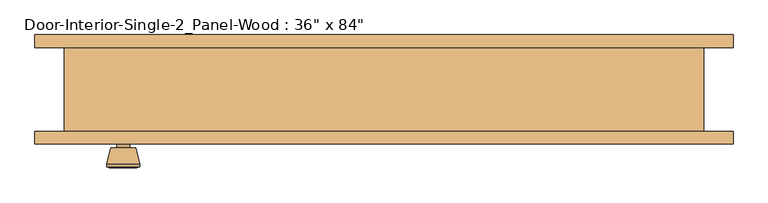
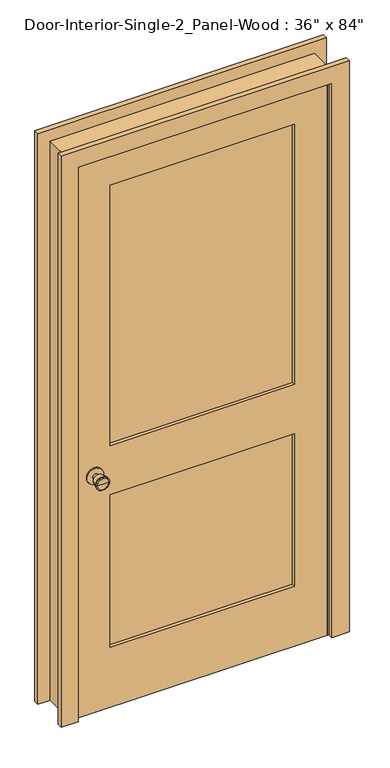
"""IFC4 building model written with IfcOpenShell, lengths in millimetres: door geometry."""

from ifc_helpers import new_model, si_unit, point, frame, frame_2d, origin, place, context, project, spatial, polyline, circle_curve, trimmed, segment, composite_curve, outline, extrude, faceted_brep, source, transform, mapped, element, save
from ifc_brep_helpers import plane_surface, cylinder_surface, revolved_surface, advanced_brep


def door_2e56f206(model_context):
    return source(origin(), model_context, "Body", "SolidModel", [
        advanced_brep(
        [(-393.7, -19.4, 914.4), (-403.7, -19.4, 914.4), (-383.7, -19.4, 914.4), (-373.2241324, 29.6, 914.4), (-414.1758676, 29.6, 914.4), (-393.7, 29.6, 914.4), (-368.7, 27.7721319, 914.4), (-418.7, 27.7721319, 914.4), (-368.7, 24.3084537, 914.4), (-418.7, 24.3084537, 914.4), (-375.063764, -0.4, 914.4), (-412.336236, -0.4, 914.4), (-383.7, -0.4, 914.4), (-403.7, -0.4, 914.4)],
        [
            (0, 1),
            (1, 2, circle_curve(frame((-393.7, -19.4, 914.4), z_axis=(0.0, -1.0, 0.0), x_axis=(-1.0, 0.0, 0.0)), 10.0)),
            (2, 0),
            (2, 1, circle_curve(frame((-393.7, -19.4, 914.4), z_axis=(0.0, -1.0, 0.0), x_axis=(-1.0, 0.0, 0.0)), 10.0)),
            (3, 4, circle_curve(frame((-393.7, 29.6, 914.4), z_axis=(0.0, 1.0, 0.0), x_axis=(-1.0, 0.0, 0.0)), 20.4758676)),
            (4, 5),
            (5, 3),
            (4, 3, circle_curve(frame((-393.7, 29.6, 914.4), z_axis=(0.0, 1.0, 0.0), x_axis=(-1.0, 0.0, 0.0)), 20.4758676)),
            (6, 7, circle_curve(frame((-393.7, 27.7721319, 914.4), z_axis=(0.0, 1.0, 0.0), x_axis=(-1.0, 0.0, 0.0)), 25.0)),
            (7, 4),
            (3, 6),
            (7, 6, circle_curve(frame((-393.7, 27.7721319, 914.4), z_axis=(0.0, 1.0, 0.0), x_axis=(-1.0, 0.0, 0.0)), 25.0)),
            (8, 9, circle_curve(frame((-393.7, 24.3084537, 914.4), z_axis=(0.0, 1.0, 0.0), x_axis=(-1.0, 0.0, 0.0)), 25.0)),
            (9, 7),
            (6, 8),
            (9, 8, circle_curve(frame((-393.7, 24.3084537, 914.4), z_axis=(0.0, 1.0, 0.0), x_axis=(-1.0, 0.0, 0.0)), 25.0)),
            (10, 11, circle_curve(frame((-393.7, -0.4, 914.4), z_axis=(0.0, 1.0, 0.0), x_axis=(-1.0, 0.0, 0.0)), 18.636236)),
            (11, 9),
            (8, 10),
            (11, 10, circle_curve(frame((-393.7, -0.4, 914.4), z_axis=(0.0, 1.0, 0.0), x_axis=(-1.0, 0.0, 0.0)), 18.636236)),
            (12, 13, circle_curve(frame((-393.7, -0.4, 914.4), z_axis=(0.0, 1.0, 0.0), x_axis=(-1.0, 0.0, 0.0)), 10.0)),
            (13, 11),
            (10, 12),
            (13, 12, circle_curve(frame((-393.7, -0.4, 914.4), z_axis=(0.0, 1.0, 0.0), x_axis=(-1.0, 0.0, 0.0)), 10.0)),
            (1, 13),
            (12, 2),
        ],
        [
            plane_surface(frame((-393.7, -19.4, 914.4), z_axis=(0.0, -1.0, 0.0), x_axis=(-1.0, 0.0, 0.0))),
            plane_surface(frame((-393.7, 29.6, 914.4), z_axis=(0.0, 1.0, 0.0), x_axis=(-1.0, 0.0, 0.0))),
            revolved_surface(polyline([(-414.1758676, 29.6, 914.4), (-418.7, 27.7721319, 914.4)]), (-393.7, -19.4, 914.4), (0.0, -1.0, 0.0)),
            cylinder_surface(frame((-393.7, -19.4, 914.4), z_axis=(0.0, -1.0, 0.0), x_axis=(-1.0, 0.0, 0.0)), 25.0),
            revolved_surface(polyline([(-418.7, 24.3084537, 914.4), (-412.336236, -0.4, 914.4)]), (-393.7, -19.4, 914.4), (0.0, -1.0, 0.0)),
            plane_surface(frame((-393.7, -0.4, 914.4), z_axis=(0.0, -1.0, 0.0), x_axis=(-1.0, 0.0, 0.0))),
            cylinder_surface(frame((-393.7, -19.4, 914.4), z_axis=(0.0, -1.0, 0.0), x_axis=(-1.0, 0.0, 0.0)), 10.0),
        ],
        [
            (0, [[1, 2, 3]]),
            (0, [[-3, 4, -1]]),
            (1, [[5, 6, 7]]),
            (1, [[8, -7, -6]]),
            (2, [[9, 10, -5, 11]]),
            (2, [[12, -11, -8, -10]]),
            (3, [[13, 14, -9, 15]]),
            (3, [[16, -15, -12, -14]]),
            (4, [[17, 18, -13, 19]]),
            (4, [[20, -19, -16, -18]]),
            (5, [[21, 22, -17, 23]]),
            (5, [[24, -23, -20, -22]]),
            (6, [[-2, 25, -21, 26]]),
            (6, [[-4, -26, -24, -25]]),
        ],
    ),
        extrude(outline(composite_curve([segment(trimmed(circle_curve(frame_2d((914.4, -393.7)), 30.0), [point((914.4, -423.7))], [point((914.4, -363.7))], False, "CARTESIAN"), True, "CONTINUOUS"), segment(trimmed(circle_curve(frame_2d((914.4, -393.7)), 30.0), [point((914.4, -363.7))], [point((914.4, -423.7))], False, "CARTESIAN"), True, "CONTINUOUS")], self_intersect=False)), frame((0.0, -25.4, 0.0), z_axis=(0.0, 1.0, 0.0), x_axis=(0.0, 0.0, 1.0)), (0.0, 0.0, 1.0), 6.0),
        advanced_brep(
        [(-393.7, -66.325, 914.4), (-383.7, -66.325, 914.4), (-403.7, -66.325, 914.4), (-373.2241324, -115.325, 914.4), (-393.7, -115.325, 914.4), (-414.1758676, -115.325, 914.4), (-368.7, -113.4971319, 914.4), (-418.7, -113.4971319, 914.4), (-368.7, -110.0334537, 914.4), (-418.7, -110.0334537, 914.4), (-375.063764, -85.325, 914.4), (-412.336236, -85.325, 914.4), (-383.7, -85.325, 914.4), (-403.7, -85.325, 914.4)],
        [
            (0, 1),
            (1, 2, circle_curve(frame((-393.7, -66.325, 914.4), z_axis=(0.0, 1.0, 0.0), x_axis=(-1.0, 0.0, 0.0)), 10.0)),
            (2, 0),
            (2, 1, circle_curve(frame((-393.7, -66.325, 914.4), z_axis=(0.0, 1.0, 0.0), x_axis=(-1.0, 0.0, 0.0)), 10.0)),
            (3, 4),
            (4, 5),
            (5, 3, circle_curve(frame((-393.7, -115.325, 914.4), z_axis=(0.0, -1.0, 0.0), x_axis=(-1.0, 0.0, 0.0)), 20.4758676)),
            (3, 5, circle_curve(frame((-393.7, -115.325, 914.4), z_axis=(0.0, -1.0, 0.0), x_axis=(-1.0, 0.0, 0.0)), 20.4758676)),
            (6, 3),
            (5, 7),
            (7, 6, circle_curve(frame((-393.7, -113.4971319, 914.4), z_axis=(0.0, -1.0, 0.0), x_axis=(-1.0, 0.0, 0.0)), 25.0)),
            (6, 7, circle_curve(frame((-393.7, -113.4971319, 914.4), z_axis=(0.0, -1.0, 0.0), x_axis=(-1.0, 0.0, 0.0)), 25.0)),
            (8, 6),
            (7, 9),
            (9, 8, circle_curve(frame((-393.7, -110.0334537, 914.4), z_axis=(0.0, -1.0, 0.0), x_axis=(-1.0, 0.0, 0.0)), 25.0)),
            (8, 9, circle_curve(frame((-393.7, -110.0334537, 914.4), z_axis=(0.0, -1.0, 0.0), x_axis=(-1.0, 0.0, 0.0)), 25.0)),
            (10, 8),
            (9, 11),
            (11, 10, circle_curve(frame((-393.7, -85.325, 914.4), z_axis=(0.0, -1.0, 0.0), x_axis=(-1.0, 0.0, 0.0)), 18.636236)),
            (10, 11, circle_curve(frame((-393.7, -85.325, 914.4), z_axis=(0.0, -1.0, 0.0), x_axis=(-1.0, 0.0, 0.0)), 18.636236)),
            (12, 10),
            (11, 13),
            (13, 12, circle_curve(frame((-393.7, -85.325, 914.4), z_axis=(0.0, -1.0, 0.0), x_axis=(-1.0, 0.0, 0.0)), 10.0)),
            (12, 13, circle_curve(frame((-393.7, -85.325, 914.4), z_axis=(0.0, -1.0, 0.0), x_axis=(-1.0, 0.0, 0.0)), 10.0)),
            (1, 12),
            (13, 2),
        ],
        [
            plane_surface(frame((-393.7, -66.325, 914.4), z_axis=(0.0, 1.0, 0.0), x_axis=(-1.0, 0.0, 0.0))),
            plane_surface(frame((-393.7, -115.325, 914.4), z_axis=(0.0, -1.0, 0.0), x_axis=(-1.0, 0.0, 0.0))),
            revolved_surface(polyline([(-414.1758676, -115.325, 914.4), (-418.7, -113.4971319, 914.4)]), (-393.7, -66.325, 914.4), (0.0, 1.0, 0.0)),
            cylinder_surface(frame((-393.7, -66.325, 914.4), z_axis=(0.0, 1.0, 0.0), x_axis=(-1.0, 0.0, 0.0)), 25.0),
            revolved_surface(polyline([(-418.7, -110.0334537, 914.4), (-412.336236, -85.325, 914.4)]), (-393.7, -66.325, 914.4), (0.0, 1.0, 0.0)),
            plane_surface(frame((-393.7, -85.325, 914.4), z_axis=(0.0, 1.0, 0.0), x_axis=(-1.0, 0.0, 0.0))),
            cylinder_surface(frame((-393.7, -66.325, 914.4), z_axis=(0.0, 1.0, 0.0), x_axis=(-1.0, 0.0, 0.0)), 10.0),
        ],
        [
            (0, [[1, 2, 3]]),
            (0, [[-3, 4, -1]]),
            (1, [[5, 6, 7]]),
            (1, [[-6, -5, 8]]),
            (2, [[9, -7, 10, 11]]),
            (2, [[-10, -8, -9, 12]]),
            (3, [[13, -11, 14, 15]]),
            (3, [[-14, -12, -13, 16]]),
            (4, [[17, -15, 18, 19]]),
            (4, [[-18, -16, -17, 20]]),
            (5, [[21, -19, 22, 23]]),
            (5, [[-22, -20, -21, 24]]),
            (6, [[25, -23, 26, -2]]),
            (6, [[-26, -24, -25, -4]]),
        ],
    ),
        extrude(outline(composite_curve([segment(trimmed(circle_curve(frame_2d((914.4, -393.7)), 30.0), [point((914.4, -423.7))], [point((914.4, -363.7))], False, "CARTESIAN"), True, "CONTINUOUS"), segment(trimmed(circle_curve(frame_2d((914.4, -393.7)), 30.0), [point((914.4, -363.7))], [point((914.4, -423.7))], False, "CARTESIAN"), True, "CONTINUOUS")], self_intersect=False)), frame((0.0, -66.325, 0.0), z_axis=(0.0, 1.0, 0.0), x_axis=(0.0, 0.0, 1.0)), (0.0, 0.0, 1.0), 6.0),
        faceted_brep([(482.6, -60.325, 0.0), (457.2, -60.325, 0.0), (457.2, -25.4, 0.0), (444.5, -25.4, 0.0), (444.5, 9.525, 0.0), (457.2, 9.525, 0.0), (457.2, 66.675, 0.0), (482.6, 66.675, 0.0), (482.6, 66.675, 2159.0), (482.6, -60.325, 2159.0), (457.2, 66.675, 2133.6), (-457.2, 66.675, 2133.6), (-457.2, 66.675, 0.0), (-482.6, 66.675, 0.0), (-482.6, 66.675, 2159.0), (457.2, 9.525, 2133.6), (444.5, 9.525, 2120.9), (-444.5, 9.525, 2120.9), (-444.5, 9.525, 0.0), (-457.2, 9.525, 0.0), (-457.2, 9.525, 2133.6), (444.5, -25.4, 2120.9), (457.2, -25.4, 2133.6), (-457.2, -25.4, 2133.6), (-457.2, -25.4, 0.0), (-444.5, -25.4, 0.0), (-444.5, -25.4, 2120.9), (457.2, -60.325, 2133.6), (-482.6, -60.325, 2159.0), (-482.6, -60.325, 0.0), (-457.2, -60.325, 0.0), (-457.2, -60.325, 2133.6)], [[[0, 1, 2, 3, 4, 5, 6, 7]], [[7, 8, 9, 0]], [[6, 10, 11, 12, 13, 14, 8, 7]], [[5, 15, 10, 6]], [[4, 16, 17, 18, 19, 20, 15, 5]], [[3, 21, 16, 4]], [[2, 22, 23, 24, 25, 26, 21, 3]], [[1, 27, 22, 2]], [[0, 9, 28, 29, 30, 31, 27, 1]], [[8, 14, 28, 9]], [[15, 20, 11, 10]], [[21, 26, 17, 16]], [[27, 31, 23, 22]], [[29, 13, 12, 19, 18, 25, 24, 30]], [[14, 13, 29, 28]], [[20, 19, 12, 11]], [[26, 25, 18, 17]], [[31, 30, 24, 23]]]),
        extrude(outline(polyline([(2133.6, -457.2), (0.0, -457.2), (0.0, 457.2), (2133.6, 457.2), (2133.6, -457.2)]), holes=[polyline([(2014.5375, -336.55), (2014.5375, 336.55), (1009.65, 336.55), (1009.65, -336.55), (2014.5375, -336.55)]), polyline([(819.15, -336.55), (819.15, 336.55), (231.775, 336.55), (231.775, -336.55), (819.15, -336.55)])]), frame((0.0, -60.325, 0.0), z_axis=(0.0, 1.0, 0.0), x_axis=(0.0, 0.0, 1.0)), (0.0, 0.0, 1.0), 34.925),
        extrude(outline(polyline([(336.55, -37.0416667), (336.55, -48.6833333), (-336.55, -48.6833333), (-336.55, -37.0416667), (336.55, -37.0416667)])), frame((0.0, 0.0, 1009.65), z_axis=(0.0, 0.0, 1.0), x_axis=(1.0, 0.0, 0.0)), (0.0, 0.0, 1.0), 1004.8875),
        extrude(outline(polyline([(336.55, -37.0416667), (336.55, -48.6833333), (-336.55, -48.6833333), (-336.55, -37.0416667), (336.55, -37.0416667)])), frame((0.0, 0.0, 231.775), z_axis=(0.0, 0.0, 1.0), x_axis=(1.0, 0.0, 0.0)), (0.0, 0.0, 1.0), 587.375),
        extrude(outline(polyline([(0.0, 527.05), (2203.45, 527.05), (2203.45, -527.05), (0.0, -527.05), (0.0, -463.55), (2139.95, -463.55), (2139.95, 463.55), (0.0, 463.55), (0.0, 527.05)])), frame((0.0, -79.375, 0.0), z_axis=(0.0, 1.0, 0.0), x_axis=(0.0, 0.0, 1.0)), (0.0, 0.0, 1.0), 19.05),
        extrude(outline(polyline([(0.0, 527.05), (2203.45, 527.05), (2203.45, -527.05), (0.0, -527.05), (0.0, -463.55), (2139.95, -463.55), (2139.95, 463.55), (0.0, 463.55), (0.0, 527.05)])), frame((0.0, 66.675, 0.0), z_axis=(0.0, 1.0, 0.0), x_axis=(0.0, 0.0, 1.0)), (0.0, 0.0, 1.0), 19.05),
    ])


if __name__ == "__main__":
    model = new_model("IFC4")
    model_context = context("Model", 3, world=origin())
    ifc_project = project(units=[si_unit("LENGTHUNIT", "METRE", prefix="MILLI")], contexts=[model_context])
    site = spatial("IfcSite", under=ifc_project)
    building = spatial("IfcBuilding", under=site)
    placement = place(None, origin())
    door_shape = door_2e56f206(model_context)
    element("IfcDoor", 1, ObjectType="Door-Interior-Single-2_Panel-Wood : 36\" x 84\"", at=placement, inside=building, context=model_context, shape_type="MappedRepresentation", body=[
        mapped(door_shape, transform((0.0, 0.0, 0.0), x_axis=(1.0, 0.0, 0.0), y_axis=(0.0, 1.0, 0.0), z_axis=(0.0, 0.0, 1.0))),
    ])
    save(model, "model.ifc")

# Revit data of these elements
# Type "Door-Interior-Single-2_Panel-Wood : 36\" x 84\""
#   Type Mark = "8"
#   Assembly Code = "C1020300"
#   Analytic Construction = "Wooden"
#   Top Rail = 0' - 4 11/16"
#   Thickness = 0' - 1 3/8"
#   Thermal Resistance (R) = 2.5876 (h·ft²·°F)/BTU
#   Swing Angle [instance default] = 90.00°
#   Stiles = 0' - 4 3/4"
#   Rough Width = 3' - 2"
#   Rough Height = 7' - 1"
#   Lock Rail = 0' - 7 1/2"
#   Height = 7' - 0"
#   Width = 3' - 0"
#   Heat Transfer Coefficient (U) = 0.3865 BTU/(h·ft²·°F)
#   Bottom Rail = 0' - 9 1/8"
#   Trim Material = Cherry
#   Panel Material = Cherry
#   Frame Material = Cherry
#   Door Handle Material = Aluminum
#   Visual Light Transmittance = 0
#   Solar Heat Gain Coefficient = 0
#   Wall Closure = (empty or 0)
#   Function = (empty or 0)
# Element 1 (IfcDoor, "Door-Interior-Single-2_Panel-Wood : 36\" x 84\"")
#   Materials on its faces: "Cherry", "Aluminum"
# Materials
#   "Cherry": class "Wood", colour RGB 226 177 128, transparency 0, Description = "Prunus Serotina", Cost = 0
#   "Aluminum": class "Metal", colour RGB 247 247 247, transparency 0, Description = "Aluminum 6061", Cost = 0
